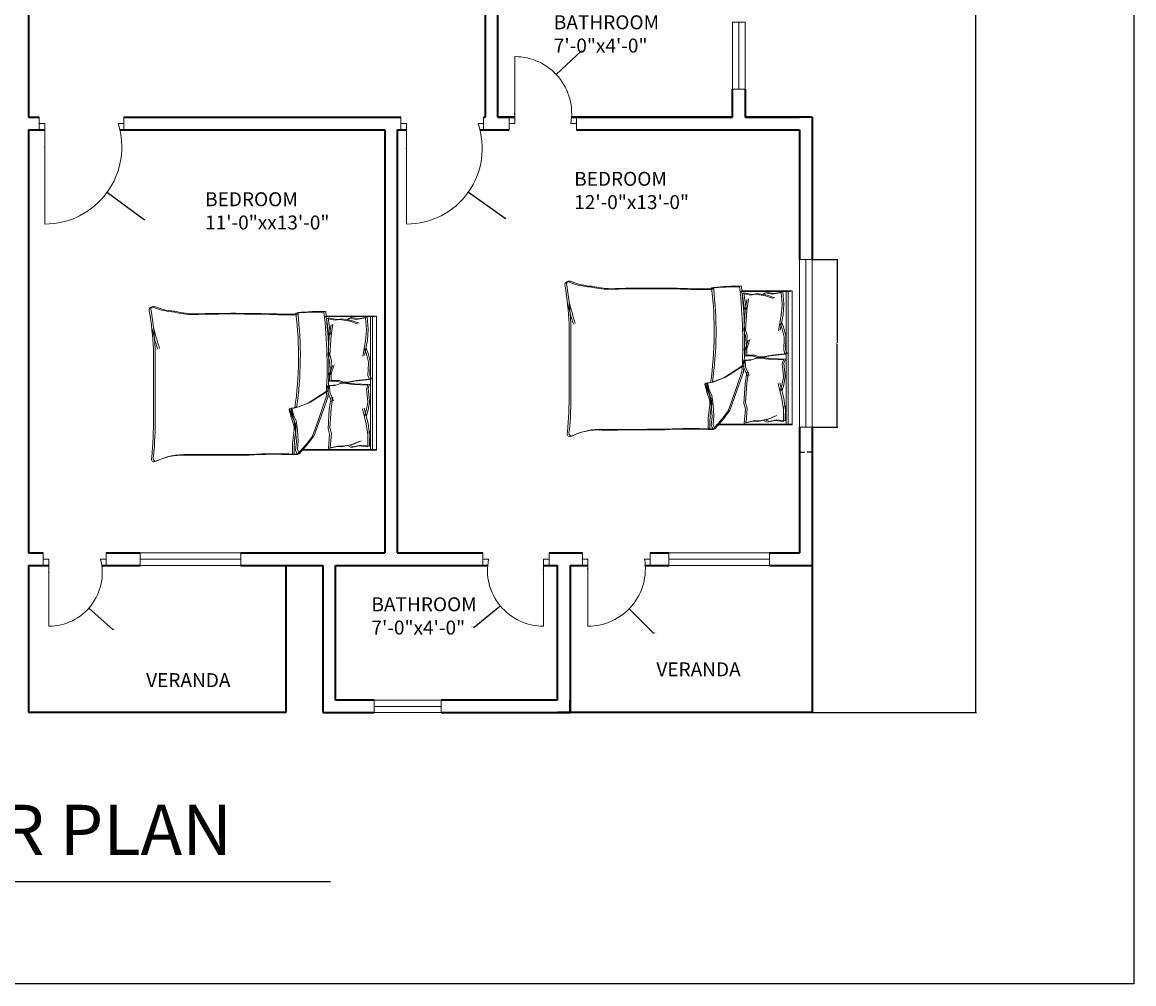
# Model space of a CAD drawing. Units: inches. Extents: x 2163 to 2982, y 1024 to 2288.
# Tile 5 of 22: x 2585 to 2982, y 1046 to 1390. Entities that reach past the tile are written whole.
import ezdxf

# ---------------------------------------------------------------- set-up
doc = ezdxf.new("R2010")
doc.units = ezdxf.units.IN
for name, color, linetype, lineweight in [('A-ANNO-DIMS', 2, 'Continuous', 18), ('A-ANNO-TTLB', 7, 'Continuous', 25), ('A-AREA-IDEN', 7, 'Continuous', 18), ('A-DOOR', 11, 'Continuous', 18), ('A-FURN', 8, 'Continuous', 13), ('A-GLAZ', 161, 'Continuous', 18), ('A-WALL', 7, 'Continuous', 35)]:
    doc.layers.add(name, color=color, linetype=linetype, lineweight=lineweight)
doc.styles.get("Standard").update_dxf_attribs({"font": 'arial.ttf'})
doc.dimstyles.get("Standard").update_dxf_attribs({"dimtxt": 0.18, "dimasz": 0.18, "dimexe": 0.18, "dimexo": 0.0625, "dimgap": 0.09, "dimtad": 0, "dimtih": 1, "dimtoh": 1, "dimdec": 4, "dimzin": 0, "dimdsep": 46, "dimtxsty": 'Standard', "dimcen": 0.09, "dimadec": 0, "dimazin": 0, "dimtfac": 1, "dimtdec": 4, "dimtofl": 0, "dimtmove": 0, "dimatfit": 3, "dimfxl": 1, "dimtolj": 1, "dimtzin": 0, "dimarcsym": 0})

# ---------------------------------------------------------------- blocks, each defined once
blk = doc.blocks.new('BED-DOUBLE')
for p, q in [((27.75, 52.87), (24.5, 49.16)), ((27.75, 52.87), (24.5, 49.16)), ((28.38, 53.1), (25.13, 49.39)), ((28.38, 53.1), (25.13, 49.39)), ((29.49, 52.95), (27.75, 52.87, 3.87)), ((29.49, 52.95), (27.75, 52.87, 3.87)), ((28.36, 51.33), (27.75, 52.87)), ((28.36, 51.33), (27.75, 52.87)), ((30.13, 53.18), (28.38, 53.1, 3.87)), ((29, 51.56), (28.38, 53.1)), ((30.13, 53.18), (28.38, 53.1, 3.87)), ((29, 51.56), (28.38, 53.1)), ((0, 51.49), (0.64, 51.49)), ((0, 3.47), (0, 51.49)), ((0, 51.27), (26.61, 51.27)), ((0, 51.27), (26.61, 51.27)), ((0.64, 51.49), (27.25, 51.49)), ((0.64, 51.49), (27.25, 51.49)), ((1.53, 3.48), (1.53, 51.27)), ((1.53, 3.47), (1.53, 51.27)), ((2.17, 3.7), (2.17, 51.49)), ((2.17, 3.7), (2.17, 51.49)), ((2.56, 50.11), (2.46, 44.71)), ((2.56, 50.11), (2.46, 44.71)), ((2.56, 50.11), (5.77, 49.73)), ((2.56, 50.11), (5.77, 49.73)), ((3.2, 50.34), (3.1, 44.94)), ((3.2, 50.34), (3.1, 44.94)), ((3.2, 50.34), (6.41, 49.96)), ((3.2, 50.34), (6.41, 49.96)), ((8.26, 49.31), (5.58, 48.13)), ((8.26, 49.31), (5.58, 48.13)), ((5.77, 49.73), (8.34, 50.33)), ((5.77, 49.73), (8.34, 50.33)), ((8.9, 49.54), (6.22, 48.36)), ((8.9, 49.54), (6.22, 48.36)), ((6.41, 49.96), (8.98, 50.56)), ((6.41, 49.96), (8.98, 50.56)), ((11.83, 50.11), (8.26, 49.31)), ((11.83, 50.11), (8.26, 49.31)), ((8.34, 50.33), (9.38, 49.81)), ((8.34, 50.33), (9.38, 49.81)), ((12.47, 50.34), (8.9, 49.54)), ((12.47, 50.34), (8.9, 49.54)), ((8.98, 50.56), (10.02, 50.04)), ((8.98, 50.56), (10.02, 50.04)), ((13.43, 49.92), (11.83, 50.11)), ((13.43, 49.92), (11.83, 50.11)), ((14.07, 50.15), (12.47, 50.34)), ((14.07, 50.15), (12.47, 50.34)), ((16.57, 50.7), (13.43, 49.92)), ((16.57, 50.7), (13.43, 49.92)), ((17.21, 50.93), (14.07, 50.15)), ((17.21, 50.93), (14.07, 50.15)), ((16.17, 45.57), (16.57, 50.7)), ((16.17, 45.57), (16.57, 50.7)), ((16.81, 45.79), (17.21, 50.93)), ((16.81, 45.79), (17.21, 50.93)), ((24.5, 49.16), (22.33, 46.22)), ((24.5, 49.16), (22.33, 46.22)), ((25.13, 49.39), (22.97, 46.45)), ((25.13, 49.39), (22.97, 46.45)), ((28.06, 48.23), (28.36, 51.33)), ((28.06, 48.23), (28.36, 51.33)), ((28.36, 44.36), (28.06, 48.23)), ((28.36, 44.36), (28.06, 48.23)), ((28.69, 48.46), (29, 51.56)), ((28.69, 48.46), (29, 51.56)), ((29, 44.59), (28.69, 48.46)), ((29, 44.59), (28.69, 48.46)), ((2.46, 44.71), (2.54, 45.71)), ((2.46, 44.71), (2.54, 45.71)), ((2.54, 45.71), (3.07, 41.91)), ((2.54, 45.71), (3.07, 41.91)), ((3.1, 44.94), (3.18, 45.94)), ((3.1, 44.94), (3.18, 45.94)), ((3.18, 45.94), (3.71, 42.14)), ((3.18, 45.94), (3.71, 42.14)), ((16.73, 43.61), (16.17, 45.57)), ((16.73, 43.61), (16.17, 45.57)), ((17.37, 43.83), (16.81, 45.79)), ((17.37, 43.83), (16.81, 45.79)), ((16.93, 36.82), (17.37, 43.83)), ((16.93, 36.82), (17.37, 43.83)), ((22.33, 46.22), (20.32, 40.64)), ((22.33, 46.22), (20.32, 40.64)), ((22.97, 46.45), (20.96, 40.87)), ((22.97, 46.45), (20.96, 40.87)), ((28.83, 40.95), (28.36, 44.36)), ((28.83, 40.95), (28.36, 44.36)), ((29.47, 41.18), (29, 44.59)), ((29.47, 41.18), (29, 44.59)), ((3.07, 41.91), (4.42, 36.49)), ((3.07, 41.91), (4.42, 36.49)), ((3.71, 42.14), (5.06, 36.72)), ((3.71, 42.14), (5.06, 36.72)), ((16.29, 36.6), (16.73, 43.61)), ((16.29, 36.6), (16.73, 43.61)), ((20.32, 40.64), (17.38, 32.31)), ((20.32, 40.64), (17.38, 32.31)), ((20.96, 40.87), (18.02, 32.53)), ((20.96, 40.87), (18.02, 32.53)), ((29.76, 38.94), (28.83, 40.95)), ((29.76, 38.94), (28.83, 40.95)), ((30.4, 39.17), (29.47, 41.18)), ((30.4, 39.17), (29.47, 41.18)), ((79.88, 15.29), (79.88, 39.91)), ((79.88, 15.29), (79.88, 39.91)), ((3.08, 37.14), (2.54, 34.2)), ((3.08, 37.13), (2.54, 34.2)), ((3.67, 39.2), (3.08, 37.14)), ((3.67, 39.2), (3.08, 37.13)), ((3.72, 37.36), (3.18, 34.43)), ((3.72, 37.36), (3.18, 34.43)), ((4.31, 39.43), (3.72, 37.36)), ((4.31, 39.43), (3.72, 37.36)), ((15.63, 32.56), (16.29, 36.6)), ((15.63, 32.56), (16.29, 36.6)), ((16.27, 32.79), (16.93, 36.82)), ((16.27, 32.79), (16.93, 36.82)), ((23.88, 34.45), (28.36, 36.15)), ((23.88, 34.45), (28.36, 36.15)), ((24.52, 34.68), (29, 36.38)), ((24.52, 34.68), (29, 36.38)), ((28.36, 36.15), (30.38, 36.46)), ((28.36, 36.15), (30.38, 36.46)), ((29, 36.38), (31.02, 36.69)), ((29, 36.38), (31.02, 36.69)), ((30.38, 36.46), (29.76, 38.94)), ((30.38, 36.46), (29.76, 38.94)), ((31.02, 36.69), (30.4, 39.17)), ((31.02, 36.69), (30.4, 39.17)), ((79.24, 15.06), (79.24, 39.68)), ((79.24, 15.06), (79.24, 39.68)), ((2.54, 34.2), (2.56, 33.88)), ((2.54, 34.2), (2.56, 33.88)), ((2.56, 33.88), (2.98, 29.46)), ((2.56, 33.88), (2.98, 29.46)), ((3.18, 34.43), (3.2, 34.11)), ((3.18, 34.43), (3.2, 34.11)), ((3.2, 34.11), (3.62, 29.68)), ((3.2, 34.11), (3.62, 29.68)), ((16.74, 30.75), (15.45, 33.82)), ((16.74, 30.75), (15.45, 33.82)), ((17.38, 30.98), (16.09, 34.05)), ((17.38, 30.98), (16.09, 34.05)), ((17.38, 30.26), (23.88, 34.45)), ((17.38, 30.26), (23.88, 34.45)), ((18.02, 30.49), (24.52, 34.68)), ((18.02, 30.49), (24.52, 34.68)), ((2.98, 29.46), (2.49, 27.98)), ((2.98, 29.46), (2.49, 27.98)), ((2.49, 27.98), (7.87, 27.73)), ((2.49, 27.98), (7.87, 27.73)), ((3.62, 29.68), (3.13, 28.21)), ((3.62, 29.68), (3.13, 28.2)), ((3.13, 28.21), (8.51, 27.96)), ((3.13, 28.2), (8.51, 27.96)), ((8.51, 27.96), (11.72, 27.58)), ((8.51, 27.96), (11.72, 27.58)), ((12.38, 27.44), (14.22, 28.13)), ((12.38, 27.44), (14.22, 28.13)), ((13.02, 27.66), (14.86, 28.36)), ((13.02, 27.66), (14.86, 28.36)), ((14.22, 28.13), (16.89, 28.3)), ((14.22, 28.13), (16.89, 28.3)), ((14.86, 28.36), (17.53, 28.53)), ((14.86, 28.36), (17.53, 28.53)), ((16.89, 28.3), (16.74, 30.75)), ((16.89, 28.3), (16.74, 30.75)), ((17.53, 28.53), (17.38, 30.98)), ((17.53, 28.53), (17.38, 30.98)), ((1.87, 25.98), (7.22, 26.56)), ((1.87, 25.98), (7.22, 26.56)), ((2.45, 24.54), (1.87, 25.98)), ((2.45, 24.54), (1.87, 25.98)), ((2.3, 20.09), (2.45, 24.54)), ((2.3, 20.09), (2.45, 24.54)), ((2.51, 26.21), (7.86, 26.79)), ((2.51, 26.21), (7.86, 26.79)), ((3.09, 24.77), (2.51, 26.21)), ((3.09, 24.77), (2.51, 26.21)), ((2.94, 20.32), (3.09, 24.77)), ((2.94, 20.32), (3.09, 24.77)), ((7.22, 26.56), (10.4, 27.14)), ((7.22, 26.56), (10.4, 27.14)), ((7.86, 26.79), (11.04, 27.37)), ((7.86, 26.79), (11.04, 27.37)), ((7.87, 27.73), (11.08, 27.35)), ((7.87, 27.73), (11.08, 27.35)), ((10.4, 27.14), (11.7, 27.14)), ((10.4, 27.14), (11.7, 27.14)), ((11.04, 27.37), (12.34, 27.37)), ((11.04, 27.37), (12.34, 27.37)), ((11.08, 27.35), (12.38, 27.44)), ((11.08, 27.35), (12.38, 27.44)), ((11.7, 27.14), (13.58, 26.56)), ((11.7, 27.14), (13.58, 26.56)), ((11.72, 27.58), (13.02, 27.66)), ((11.72, 27.58), (13.02, 27.66)), ((12.34, 27.37), (14.22, 26.79)), ((12.34, 27.37), (14.22, 26.79)), ((13.58, 26.56), (16.26, 26.56)), ((13.58, 26.56), (16.26, 26.56)), ((14.22, 26.79), (16.9, 26.79)), ((14.22, 26.79), (16.9, 26.79)), ((16.26, 24.1), (15.17, 20.96)), ((16.26, 24.1), (15.17, 20.96)), ((16.9, 24.33), (15.81, 21.19)), ((16.9, 24.33), (15.81, 21.19)), ((16.17, 19.38), (16.57, 24.52)), ((16.17, 19.38), (16.57, 24.52)), ((16.26, 26.56), (16.26, 24.1)), ((16.26, 26.56), (16.26, 24.1)), ((16.81, 19.61), (17.21, 24.74)), ((16.81, 19.61), (17.21, 24.74)), ((16.9, 26.79), (16.9, 24.33)), ((16.9, 26.79), (16.9, 24.33)), ((2.3, 19.77), (2.3, 20.09)), ((2.3, 19.77), (2.3, 20.09)), ((2.94, 20), (2.94, 20.32)), ((2.94, 20), (2.94, 20.32)), ((3.67, 17.11), (2.94, 20)), ((3.67, 17.11), (2.94, 20)), ((3.03, 16.88), (2.3, 19.77)), ((3.03, 16.88), (2.3, 19.77)), ((3.75, 14.85), (3.03, 16.88)), ((3.75, 14.85), (3.03, 16.88)), ((3.32, 12.11), (4.33, 17.6)), ((3.32, 12.11), (4.33, 17.6)), ((4.39, 15.08), (3.67, 17.11)), ((4.39, 15.08), (3.67, 17.11)), ((3.96, 12.34), (4.97, 17.83)), ((3.96, 12.34), (4.97, 17.83)), ((16.73, 17.42), (16.17, 19.38)), ((16.73, 17.42), (16.17, 19.38)), ((16.29, 10.41), (16.73, 17.42)), ((16.29, 10.41), (16.73, 17.42)), ((17.37, 17.65), (16.81, 19.61)), ((17.37, 17.65), (16.81, 19.61)), ((16.93, 10.64), (17.37, 17.65)), ((16.93, 10.64), (17.37, 17.65)), ((3.03, 8.28), (3.32, 12.11)), ((3.03, 8.28), (3.32, 12.11)), ((3.67, 8.51), (3.96, 12.34)), ((3.67, 8.51), (3.96, 12.34)), ((3.01, 8.18), (3.03, 8.28)), ((3.01, 8.18), (3.03, 8.28)), ((3.34, 3.9), (3.01, 8.18)), ((3.34, 3.9), (3.01, 8.18)), ((3.65, 8.41), (3.67, 8.51)), ((3.65, 8.41), (3.67, 8.51)), ((3.98, 4.13), (3.65, 8.41)), ((3.98, 4.13), (3.65, 8.41)), ((15.63, 6.38), (16.29, 10.41)), ((15.63, 6.38), (16.29, 10.41)), ((16.27, 6.61), (16.93, 10.64)), ((16.27, 6.61), (16.93, 10.64)), ((16.29, 10.41), (16.62, 9.28)), ((16.29, 10.41), (16.62, 9.28)), ((16.62, 9.28), (17.34, 4.18)), ((16.62, 9.28), (17.34, 4.18)), ((16.93, 10.64), (17.26, 9.51)), ((16.93, 10.64), (17.26, 9.51)), ((17.26, 9.51), (17.98, 4.41)), ((17.26, 9.51), (17.98, 4.41)), ((3.32, 3.89), (6.5, 4.47)), ((3.32, 3.89), (6.5, 4.47)), ((3.96, 4.12), (7.14, 4.7)), ((3.96, 4.12), (7.14, 4.7)), ((8.95, 5.05), (6.21, 6.06)), ((8.95, 5.05), (6.21, 6.06)), ((6.5, 4.47), (9.1, 4.04)), ((6.5, 4.47), (9.1, 4.04)), ((9.59, 5.28), (6.85, 6.29)), ((9.59, 5.28), (6.85, 6.29)), ((7.14, 4.7), (9.74, 4.27)), ((7.14, 4.7), (9.74, 4.27)), ((12.57, 4.47), (8.95, 5.05)), ((12.57, 4.47), (8.95, 5.05)), ((9.1, 4.04), (10.11, 4.62)), ((9.1, 4.04), (10.11, 4.62)), ((13.21, 4.7), (9.59, 5.28)), ((13.21, 4.7), (9.59, 5.28)), ((9.74, 4.27), (10.75, 4.85)), ((9.74, 4.27), (10.75, 4.85)), ((14.16, 4.76), (12.57, 4.47)), ((14.16, 4.76), (12.57, 4.47)), ((14.8, 4.99), (13.21, 4.7)), ((14.8, 4.99), (13.21, 4.7)), ((17.34, 4.18), (14.16, 4.76)), ((17.34, 4.18), (14.16, 4.76)), ((17.98, 4.41), (14.8, 4.99)), ((17.98, 4.41), (14.8, 4.99)), ((18.11, 3.48), (0, 3.48)), ((18.11, 3.47), (0, 3.47)), ((18.75, 3.7), (0.64, 3.7)), ((18.75, 3.7), (0.64, 3.7))]:
    blk.add_line(p, q)
for centre, radius, start, end in [((69.31, 76.39), 23.07, 267.4714, 296.4681), ((69.31, 76.39), 23.07, 267.4714, 296.4681), ((79.51, 54.64), 1.1, 332.6588, 86.02), ((79.51, 54.64), 1.1, 332.6588, 86.02), ((-6.66, 51.33), 36.18, 349.8763, 2.5657), ((-6.66, 51.33), 36.18, 349.8763, 2.5657), ((36.31, 182.27), 129.5, 266.9791, 273.8365), ((36.31, 182.27), 129.5, 266.9791, 273.8365), ((-6.02, 51.56), 36.18, 349.8763, 2.5657), ((-6.02, 51.56), 36.18, 349.8763, 2.5657), ((36.95, 182.49), 129.5, 266.9791, 273.8365), ((36.95, 182.49), 129.5, 266.9791, 273.8365), ((67.82, -4508.74), 4561.86, 90.00217, 90.28689), ((67.82, -4508.74), 4561.86, 90.00217, 90.28689), ((68.46, -4508.52), 4561.86, 90.00217, 90.28689), ((68.46, -4508.52), 4561.86, 90.00217, 90.28689), ((68.67, 76.16), 23.07, 267.4714, 296.4681), ((68.67, 76.16), 23.07, 267.4714, 296.4681), ((78.87, 54.41), 1.1, 332.6588, 86.02), ((78.87, 54.41), 1.1, 332.6588, 86.02), ((212.28, 41.15), 133.04, 174.4998, 180.6351), ((212.28, 41.15), 133.04, 174.4998, 180.6351), ((212.92, 41.38), 133.04, 174.4998, 180.6351), ((212.92, 41.38), 133.04, 174.4998, 180.6351), ((35.07, 43.74), 6.22, 168.6608, 203.7384), ((35.07, 43.74), 6.22, 168.6608, 203.7384), ((35.71, 43.97), 6.22, 168.6608, 203.7384), ((35.71, 43.97), 6.22, 168.6608, 203.7384), ((1.48, 31.15), 29.65, 10.6617, 19.8806), ((1.48, 31.15), 29.65, 10.6617, 19.8806), ((2.12, 31.38), 29.65, 10.6617, 19.8806), ((2.12, 31.38), 29.65, 10.6617, 19.8806), ((156.32, 17.76), 129.02, 171.7845, 186.9006), ((156.32, 17.76), 129.02, 171.7845, 186.9006), ((156.96, 17.98), 129.02, 171.7845, 186.9006), ((156.96, 17.98), 129.02, 171.7845, 186.9006), ((30.44, 36.64), 0.185, 250.2464, 1.1377), ((30.44, 36.64), 0.185, 250.2464, 1.1377), ((31.08, 36.86), 0.185, 250.2464, 1.1377), ((31.08, 36.86), 0.185, 250.2464, 1.1377), ((182.05, 21.36), 164.97, 176.0865, 186.7821), ((182.05, 21.36), 164.97, 176.0865, 186.7821), ((182.69, 21.59), 164.97, 176.0865, 186.7821), ((182.69, 21.59), 164.97, 176.0865, 186.7821), ((-23.71, -17.22), 106.46, 13.3832, 17.7053), ((-23.71, -17.22), 106.46, 13.3832, 17.7053), ((-23.07, -16.99), 106.46, 13.3832, 17.7053), ((-23.07, -16.99), 106.46, 13.3832, 17.7053), ((200.84, 21.43), 121.76, 182.9958, 189.4091), ((200.84, 21.43), 121.76, 182.9958, 189.4091), ((201.48, 21.66), 121.76, 182.9958, 189.4091), ((201.48, 21.65), 121.76, 182.9958, 189.4091), ((20.1, 85.16), 83.31, 268.7218, 275.604), ((20.1, 85.16), 83.31, 268.7218, 275.604), ((20.74, 85.39), 83.31, 268.7218, 275.604), ((20.74, 85.39), 83.31, 268.7218, 275.604), ((31.17, -167.31), 170.11, 88.4762, 91.0082), ((31.17, -167.31), 170.11, 88.4762, 91.0082), ((31.81, -167.08), 170.11, 88.4762, 91.0082), ((31.81, -167.08), 170.11, 88.4762, 91.0082), ((50.61, 484.82), 482.31, 268.2277, 271.7185), ((50.61, 484.82), 482.31, 268.2277, 271.7185), ((51.25, 485.05), 482.31, 268.2277, 271.7185), ((51.25, 485.05), 482.31, 268.2277, 271.7185), ((64.51, -26.9), 29.63, 76.0648, 88.9113), ((64.51, -26.9), 29.63, 76.0648, 88.9113), ((65.15, -26.67), 29.63, 76.0648, 88.9113), ((65.15, -26.67), 29.63, 76.0648, 88.9113), ((70.28, -21.66), 23.56, 67.9751, 86.652), ((70.28, -21.66), 23.56, 67.9751, 86.652), ((70.91, -21.43), 23.56, 67.9751, 86.652), ((70.91, -21.43), 23.56, 67.9751, 86.652), ((79.72, 1.09), 1.09, 236.1736, 23.4781), ((79.72, 1.09), 1.09, 236.1736, 23.4781), ((80.36, 1.32), 1.09, 236.1736, 23.4781), ((80.36, 1.32), 1.09, 236.1736, 23.4781)]:
    blk.add_arc(centre, radius, start, end)
blk = doc.blocks.new('WIN-24')
for p, q in [((0, 24), (4.5, 24)), ((0, 24), (0, 0)), ((4.5, 24), (2.25, 24)), ((2.25, 24), (2.25, 0)), ((4.5, 24), (4.5, 0)), ((2.25, 0), (0, 0)), ((0, 0), (4.5, 0))]:
    blk.add_line(p, q)
blk = doc.blocks.new('WIN-60')
for p, q in [((2.25, 60), (0, 60)), ((0, 60), (4.5, 60)), ((0, 60), (0, 0)), ((2.25, 0), (2.25, 60)), ((4.5, 60), (4.5, 0)), ((0, 0), (4.5, 0)), ((4.5, 0), (2.25, 0))]:
    blk.add_line(p, q)
blk = doc.blocks.new('WIN-36')
for p, q in [((2.25, 36), (0, 36)), ((0, 36), (4.5, 36)), ((0, 36), (0, 0)), ((2.25, 0), (2.25, 36)), ((4.5, 36), (4.5, 0)), ((0, 0), (4.5, 0)), ((4.5, 0), (2.25, 0))]:
    blk.add_line(p, q)
blk = doc.blocks.new('*D13')
at = {"layer": 'A-ANNO-DIMS', "color": 0, "lineweight": -2, "transparency": 16777216}
for p, q in [((2867.4, 1305.36), (2876.52, 1305.36)), ((2876.34, 1305.18), (2876.34, 1275.54)), ((2876.34, 1245.54), (2876.34, 1275.18)), ((2867.4, 1245.36), (2876.52, 1245.36))]:
    blk.add_line(p, q, dxfattribs=at)
at = {"layer": 'A-ANNO-DIMS', "color": 0, "transparency": 16777216}
for points in [[(2876.31, 1305.18), (2876.37, 1305.18), (2876.34, 1305.36)], [(2876.31, 1245.54), (2876.37, 1245.54), (2876.34, 1245.36)]]:
    blk.add_solid(points, dxfattribs=at)
at = {"layer": 'Defpoints', "color": 0, "transparency": 16777216}
for p in [(2867.34, 1305.36), (2876.34, 1305.36), (2867.34, 1245.36)]:
    blk.add_point(p, dxfattribs=at)
at = {"layer": 'A-ANNO-DIMS', "color": 0, "transparency": 16777216, "insert": (2876.34, 1275.36), "char_height": 0.18, "attachment_point": 5}
blk.add_mtext('\\A1;WINDOW 60 TYP.', dxfattribs=at)
blk = doc.blocks.new('*D14')
at = {"layer": 'A-ANNO-DIMS', "color": 0, "lineweight": -2, "transparency": 16777216}
for p, q in [((2862.84, 1245.3), (2862.84, 1236.18)), ((2867.34, 1245.3), (2867.34, 1236.18)), ((2863.02, 1236.36), (2864.63, 1236.36)), ((2867.16, 1236.36), (2865.55, 1236.36))]:
    blk.add_line(p, q, dxfattribs=at)
at = {"layer": 'A-ANNO-DIMS', "color": 0, "transparency": 16777216}
for points in [[(2863.02, 1236.39), (2863.02, 1236.33), (2862.84, 1236.36)], [(2867.16, 1236.39), (2867.16, 1236.33), (2867.34, 1236.36)]]:
    blk.add_solid(points, dxfattribs=at)
at = {"layer": 'Defpoints', "color": 0, "transparency": 16777216}
for p in [(2862.84, 1245.36), (2867.34, 1245.36), (2867.34, 1236.36)]:
    blk.add_point(p, dxfattribs=at)
at = {"layer": 'A-ANNO-DIMS', "color": 0, "transparency": 16777216, "insert": (2865.09, 1236.36), "char_height": 0.18, "attachment_point": 5}
blk.add_mtext('\\A1;5 TYP.', dxfattribs=at)
blk = doc.blocks.new('*D32')
at = {"layer": 'A-ANNO-DIMS', "color": 0, "lineweight": -2, "transparency": 16777216}
for p, q in [((2867.4, 2229.27), (2926.17, 2229.27)), ((2925.99, 2229.09), (2925.99, 1686.35)), ((2925.99, 1143.25), (2925.99, 1685.99)), ((2867.4, 1143.07), (2926.17, 1143.07))]:
    blk.add_line(p, q, dxfattribs=at)
at = {"layer": 'A-ANNO-DIMS', "color": 0, "transparency": 16777216}
for points in [[(2925.96, 2229.09), (2926.02, 2229.09), (2925.99, 2229.27)], [(2925.96, 1143.25), (2926.02, 1143.25), (2925.99, 1143.07)]]:
    blk.add_solid(points, dxfattribs=at)
at = {"layer": 'Defpoints', "color": 0, "transparency": 16777216}
for p in [(2867.34, 2229.27), (2925.99, 2229.27), (2867.34, 1143.07)]:
    blk.add_point(p, dxfattribs=at)
at = {"layer": 'A-ANNO-DIMS', "color": 0, "transparency": 16777216, "insert": (2925.99, 1686.17), "char_height": 0.18, "attachment_point": 5}
blk.add_mtext('\\A1;1086.2', dxfattribs=at)
blk = doc.blocks.new('*D45')
at = {"layer": 'A-ANNO-DIMS', "color": 0, "lineweight": -2, "transparency": 16777216}
for p, q in [((2592.54, 1345.61), (2592.72, 1345.61)), ((2592.63, 1345.52), (2592.63, 1345.7)), ((2628.28, 1319.58), (2615.06, 1329.24)), ((2628.46, 1319.58), (2628.28, 1319.58))]:
    blk.add_line(p, q, dxfattribs=at)
at = {"layer": 'A-ANNO-DIMS', "color": 0, "transparency": 16777216}
blk.add_solid([(2615.08, 1329.26), (2615.04, 1329.21), (2614.91, 1329.34)], dxfattribs=at)
at = {"layer": 'Defpoints', "color": 0, "transparency": 16777216}
for p in [(2592.63, 1345.61), (2614.91, 1329.34)]:
    blk.add_point(p, dxfattribs=at)
at = {"layer": 'A-ANNO-DIMS', "color": 0, "transparency": 16777216, "insert": (2628.94, 1319.58), "char_height": 0.18, "attachment_point": 5}
blk.add_mtext('\\A1;R27.59', dxfattribs=at)
blk = doc.blocks.new('*D48')
at = {"layer": 'A-ANNO-DIMS', "color": 0, "lineweight": -2, "transparency": 16777216}
for p, q in [((2722.07, 1345.1), (2722.25, 1345.1)), ((2722.16, 1345.01), (2722.16, 1345.19)), ((2757.49, 1320), (2744.39, 1329.31)), ((2757.67, 1320), (2757.49, 1320))]:
    blk.add_line(p, q, dxfattribs=at)
at = {"layer": 'A-ANNO-DIMS', "color": 0, "transparency": 16777216}
blk.add_solid([(2744.4, 1329.34), (2744.37, 1329.29), (2744.24, 1329.42)], dxfattribs=at)
at = {"layer": 'Defpoints', "color": 0, "transparency": 16777216}
for p in [(2722.16, 1345.1), (2744.24, 1329.42)]:
    blk.add_point(p, dxfattribs=at)
at = {"layer": 'A-ANNO-DIMS', "color": 0, "transparency": 16777216, "insert": (2758.22, 1320), "char_height": 0.18, "attachment_point": 5}
blk.add_mtext('\\A1;R27.086', dxfattribs=at)
blk = doc.blocks.new('*D66')
at = {"layer": 'A-ANNO-DIMS', "color": 0, "lineweight": -2, "transparency": 16777216}
for p, q in [((2594, 1193.17), (2594.18, 1193.17)), ((2594.09, 1193.08), (2594.09, 1193.26)), ((2617.05, 1172.89), (2608.58, 1180.37)), ((2617.23, 1172.89), (2617.05, 1172.89))]:
    blk.add_line(p, q, dxfattribs=at)
at = {"layer": 'A-ANNO-DIMS', "color": 0, "transparency": 16777216}
blk.add_solid([(2608.6, 1180.4), (2608.56, 1180.35), (2608.44, 1180.49)], dxfattribs=at)
at = {"layer": 'Defpoints', "color": 0, "transparency": 16777216}
for p in [(2594.09, 1193.17), (2608.44, 1180.49)]:
    blk.add_point(p, dxfattribs=at)
at = {"layer": 'A-ANNO-DIMS', "color": 0, "transparency": 16777216, "insert": (2617.72, 1172.89), "char_height": 0.18, "attachment_point": 5}
blk.add_mtext('\\A1;R19.15', dxfattribs=at)
blk = doc.blocks.new('*D67')
at = {"layer": 'A-ANNO-DIMS', "color": 0, "lineweight": -2, "transparency": 16777216}
for p, q in [((2771.13, 1194.12), (2771.31, 1194.12)), ((2771.22, 1194.03), (2771.22, 1194.21)), ((2746.35, 1173.73), (2755.54, 1181.26)), ((2746.17, 1173.73), (2746.35, 1173.73))]:
    blk.add_line(p, q, dxfattribs=at)
at = {"layer": 'A-ANNO-DIMS', "color": 0, "transparency": 16777216}
blk.add_solid([(2755.52, 1181.29), (2755.56, 1181.24), (2755.68, 1181.38)], dxfattribs=at)
at = {"layer": 'Defpoints', "color": 0, "transparency": 16777216}
for p in [(2771.22, 1194.12), (2755.68, 1181.38)]:
    blk.add_point(p, dxfattribs=at)
at = {"layer": 'A-ANNO-DIMS', "color": 0, "transparency": 16777216, "insert": (2745.62, 1173.73), "char_height": 0.18, "attachment_point": 5}
blk.add_mtext('\\A1;R20.097', dxfattribs=at)
blk = doc.blocks.new('*D68')
at = {"layer": 'A-ANNO-DIMS', "color": 0, "lineweight": -2, "transparency": 16777216}
for p, q in [((2787, 1194.57), (2787.18, 1194.57)), ((2787.09, 1194.48), (2787.09, 1194.66)), ((2810.61, 1171.58), (2801.92, 1180.08)), ((2810.79, 1171.58), (2810.61, 1171.58))]:
    blk.add_line(p, q, dxfattribs=at)
at = {"layer": 'A-ANNO-DIMS', "color": 0, "transparency": 16777216}
blk.add_solid([(2801.94, 1180.1), (2801.9, 1180.06), (2801.79, 1180.2)], dxfattribs=at)
at = {"layer": 'Defpoints', "color": 0, "transparency": 16777216}
for p in [(2787.09, 1194.57), (2801.79, 1180.2)]:
    blk.add_point(p, dxfattribs=at)
at = {"layer": 'A-ANNO-DIMS', "color": 0, "transparency": 16777216, "insert": (2811.34, 1171.58), "char_height": 0.18, "attachment_point": 5}
blk.add_mtext('\\A1;R20.556', dxfattribs=at)
blk = doc.blocks.new('*D77')
at = {"layer": 'A-ANNO-DIMS', "color": 0, "lineweight": -2, "transparency": 16777216}
for p, q in [((2784.62, 1380.01), (2775.84, 1371.74)), ((2784.8, 1380.01), (2784.62, 1380.01)), ((2760.78, 1357.62), (2760.96, 1357.62)), ((2760.87, 1357.53), (2760.87, 1357.71))]:
    blk.add_line(p, q, dxfattribs=at)
at = {"layer": 'A-ANNO-DIMS', "color": 0, "transparency": 16777216}
blk.add_solid([(2775.82, 1371.76), (2775.86, 1371.72), (2775.71, 1371.62)], dxfattribs=at)
at = {"layer": 'Defpoints', "color": 0, "transparency": 16777216}
for p in [(2775.71, 1371.62), (2760.87, 1357.62)]:
    blk.add_point(p, dxfattribs=at)
at = {"layer": 'A-ANNO-DIMS', "color": 0, "transparency": 16777216, "insert": (2785.21, 1380.01), "char_height": 0.18, "attachment_point": 5}
blk.add_mtext('\\A1;R20.4', dxfattribs=at)

msp = doc.modelspace()

# ---------------------------------------------------------------- linework, layer by layer
at = {"layer": 'A-ANNO-TTLB'}
msp.add_line((2427.5046, 1082.6234), (2694.9452, 1082.6234), dxfattribs=at)
msp.add_lwpolyline([(2162.6841, 2274.6054), (2982.469, 2274.6054), (2982.469, 1045.9691), (2162.6841, 1045.9691)], close=True, dxfattribs=at)
at = {"layer": 'A-DOOR'}
for p, q in [((2760.8716, 1354.0188), (2760.8716, 1378.0188)), ((2590.6292, 1351.7688), (2590.6292, 1356.2688)), ((2590.6292, 1356.2688), (2590.6292, 1354.0188)), ((2590.6292, 1354.0188), (2592.6292, 1354.0188)), ((2592.6292, 1354.0188), (2592.6292, 1318.0188)), ((2620.9043, 1354.0188), (2618.9043, 1354.0188)), ((2620.9043, 1356.2688), (2620.9043, 1351.7688)), ((2620.9043, 1351.7688), (2620.9043, 1354.0188)), ((2720.1594, 1351.7688), (2720.1594, 1356.2688)), ((2720.1594, 1356.2688), (2720.1594, 1354.0188)), ((2720.1594, 1354.0188), (2722.1594, 1354.0188)), ((2722.1594, 1354.0188), (2722.1594, 1318.0188)), ((2749.7366, 1354.0188), (2747.7366, 1354.0188)), ((2749.7366, 1356.2688), (2749.7366, 1351.7688)), ((2749.7366, 1351.7688), (2749.7366, 1354.0188)), ((2758.8716, 1356.2688), (2758.8716, 1351.7688)), ((2758.8716, 1351.7688), (2758.8716, 1354.0188)), ((2758.8716, 1354.0188), (2760.8716, 1354.0188)), ((2782.9533, 1354.0188), (2780.9533, 1354.0188)), ((2782.9533, 1356.2688), (2782.9533, 1351.7688)), ((2782.9533, 1351.7688), (2782.9533, 1354.0188)), ((2592.0869, 1200.2688), (2592.0869, 1195.7688)), ((2592.0869, 1195.7688), (2592.0869, 1198.0188)), ((2592.0869, 1198.0188), (2594.0869, 1198.0188)), ((2594.0869, 1198.0188), (2594.0869, 1174.0188)), ((2614.6146, 1198.0188), (2612.6146, 1198.0188)), ((2614.6146, 1200.2688), (2614.6146, 1195.7688)), ((2614.6146, 1195.7688), (2614.6146, 1198.0188)), ((2749.508, 1195.7688), (2749.508, 1200.2688)), ((2749.508, 1200.2688), (2749.508, 1198.0188)), ((2749.508, 1198.0188), (2751.508, 1198.0188)), ((2773.2218, 1198.0188), (2771.2218, 1198.0188)), ((2771.2218, 1198.0188), (2771.2218, 1174.0188)), ((2773.2218, 1195.7688), (2773.2218, 1200.2688)), ((2773.2218, 1200.2688), (2773.2218, 1198.0188)), ((2785.093, 1195.7688), (2785.093, 1200.2688)), ((2785.093, 1200.2688), (2785.093, 1198.0188)), ((2785.093, 1198.0188), (2787.093, 1198.0188)), ((2787.093, 1198.0188), (2787.093, 1174.0188)), ((2809.358, 1198.0188), (2807.358, 1198.0188)), ((2809.358, 1195.7688), (2809.358, 1200.2688)), ((2809.358, 1200.2688), (2809.358, 1198.0188))]:
    msp.add_line(p, q, dxfattribs=at)
for centre, radius, start, end in [((2760.8716, 1357.6173), 20.4016, 349.841009, 90), ((2592.6292, 1345.6075), 27.5886, 270, 17.751249), ((2722.1594, 1345.1049), 27.086, 270, 19.214067), ((2594.0869, 1193.1705), 19.1517, 270, 14.664329), ((2771.2218, 1194.1154), 20.0965, 168.799919, 270), ((2787.093, 1194.5745), 20.5557, 270, 9.646048)]:
    msp.add_arc(centre, radius, start, end, dxfattribs=at)
at = {"layer": 'A-WALL'}
for p, q in [((2586.8389, 1648.0603), (2586.8389, 1356.2688)), ((2750.3389, 1404.2688), (2750.3389, 1356.2688)), ((2754.8389, 1356.2688), (2754.8389, 1404.2688)), ((2838.8389, 1356.2688), (2838.8389, 1366.3249)), ((2843.3389, 1366.3249), (2843.3389, 1356.2688)), ((2586.8389, 1356.2688), (2590.6292, 1356.2688)), ((2620.9043, 1356.2688), (2714.3389, 1356.2688)), ((2714.3389, 1356.2688), (2720.1594, 1356.2688)), ((2749.7366, 1356.2688), (2750.3389, 1356.2688)), ((2754.8389, 1356.2688), (2760.8716, 1356.2688)), ((2760.8716, 1356.2688), (2754.8389, 1356.2688)), ((2838.8389, 1356.2688), (2781.2285, 1356.2688)), ((2781.2285, 1356.2688), (2838.8389, 1356.2688)), ((2867.3389, 1356.2688), (2843.3389, 1356.2688)), ((2843.3389, 1356.2688), (2862.8389, 1356.2688)), ((2867.3389, 1356.2688), (2867.3389, 1305.3618)), ((2586.8389, 1351.7688), (2586.8389, 1200.2688)), ((2586.8389, 1351.7688), (2592.6292, 1351.7688)), ((2619.521, 1351.7688), (2714.3389, 1351.7688)), ((2714.3389, 1351.7688), (2714.3389, 1200.2688)), ((2718.8389, 1351.7688), (2722.1594, 1351.7688)), ((2718.8389, 1351.7688), (2718.8389, 1200.2688)), ((2748.4128, 1351.7688), (2758.8716, 1351.7688)), ((2782.9533, 1351.7688), (2862.8389, 1351.7688)), ((2862.8389, 1351.7688), (2862.8389, 1305.3618)), ((2862.8389, 1245.3618), (2862.8389, 1200.2688)), ((2867.3389, 1245.3618), (2867.3389, 1195.7688)), ((2586.8389, 1200.2688), (2592.0869, 1200.2688)), ((2614.6146, 1200.2688), (2626.8098, 1200.2688)), ((2662.8098, 1200.2688), (2714.3389, 1200.2688)), ((2718.8389, 1200.2688), (2749.508, 1200.2688)), ((2773.2218, 1200.2688), (2785.093, 1200.2688)), ((2776.2464, 1200.2688), (2780.7464, 1200.2688)), ((2809.358, 1200.2688), (2816.0529, 1200.2688)), ((2852.0529, 1200.2688), (2862.8389, 1200.2688)), ((2586.8389, 1195.7688), (2586.8389, 1143.2688)), ((2586.8389, 1195.7688), (2594.0869, 1195.7688)), ((2613.0614, 1195.7688), (2626.8098, 1195.7688)), ((2662.8098, 1195.7688), (2692.2464, 1195.7688)), ((2679.0829, 1143.2688), (2679.0829, 1195.7688)), ((2692.2464, 1195.7688), (2692.2464, 1143.0732)), ((2696.7464, 1147.5732), (2696.7464, 1195.7688)), ((2696.7464, 1195.7688), (2751.1934, 1195.7688)), ((2771.2218, 1195.7688), (2776.2464, 1195.7688)), ((2776.2464, 1147.5732), (2776.2464, 1195.7688)), ((2780.7464, 1195.7688), (2780.7464, 1143.0732)), ((2780.7464, 1195.7688), (2787.093, 1195.7688)), ((2807.6139, 1195.7688), (2816.0529, 1195.7688)), ((2852.0529, 1195.7688), (2867.3389, 1195.7688)), ((2867.3389, 1195.7688), (2867.3389, 1143.0732)), ((2710.5865, 1147.5732), (2696.7464, 1147.5732)), ((2776.2464, 1147.5732), (2734.5865, 1147.5732)), ((2780.7464, 1143.0732), (2780.7464, 1147.5732)), ((2586.8389, 1143.2688), (2679.0829, 1143.2688)), ((2692.2464, 1143.0732), (2710.5865, 1143.0732)), ((2734.5865, 1143.0732), (2776.2464, 1143.0732)), ((2780.7464, 1143.0732), (2776.2464, 1143.0732)), ((2776.2464, 1143.0732), (2780.7464, 1143.0732)), ((2867.3389, 1143.0732), (2780.7464, 1143.0732))]:
    msp.add_line(p, q, dxfattribs=at)

# ---------------------------------------------------------------- block references
at = {"layer": 'A-FURN', "rotation": 180}
for p in [(2860.2409, 1297.626), (2711.4412, 1288.5851)]:
    msp.add_blockref('BED-DOUBLE', p, dxfattribs=at)
at = {"layer": 'A-GLAZ', "extrusion": (0, 0, -1), "zscale": -1}
for p, rotation in [((-2838.839, 1390.3245), 180), ((-2710.587, 1143.0733), 90)]:
    msp.add_blockref('WIN-24', p, dxfattribs=dict(at, rotation=rotation))
at = {"layer": 'A-GLAZ'}
msp.add_blockref('WIN-60', (2862.839, 1245.3618), dxfattribs=at)
at = {"layer": 'A-GLAZ', "rotation": 270}
for p in [(2626.8094, 1200.2688), (2816.0525, 1200.2688)]:
    msp.add_blockref('WIN-36', p, dxfattribs=at)

# ---------------------------------------------------------------- texts
at = {"layer": 'A-ANNO-TTLB', "insert": (2442.4425, 1110.0829), "char_height": 18, "attachment_point": 1}
msp.add_mtext_dynamic_manual_height_columns('FIRST FLOOR PLAN', width=728.99492, gutter_width=12.5, heights=[0], dxfattribs=at)
at = {"layer": 'A-AREA-IDEN', "char_height": 5, "attachment_point": 1}
for s, width, insert in [('BATHROOM\\P7\'-0"x4\'-0"', 52.770015, (2774.8723, 1392.7938)), ('BEDROOM\\P12\'-0"x13\'-0"', 62.207874, (2782.1606, 1336.7403)), ('BEDROOM\\P11\'-0"xx13\'-0"', 110.183291, (2650.0452, 1329.4297)), ('BATHROOM\\P7\'-0"x4\'-0"', 77.436959, (2709.5926, 1184.369)), ('VERANDA', 68.460367, (2811.5789, 1161.0749)), ('VERANDA', 53.947048, (2628.9428, 1157.2097))]:
    msp.add_mtext_dynamic_manual_height_columns(s, width=width, gutter_width=12.5, heights=[0], dxfattribs=dict(at, insert=insert))

# ---------------------------------------------------------------- dimensions: what is measured, and where the dimension line sits
at = {"layer": 'A-ANNO-DIMS'}
dim = msp.add_linear_dim(base=(2925.9889, 2229.2688), p1=(2867.3389, 1143.0732), p2=(2867.3389, 2229.2688), angle=90, dimstyle='Standard', override={"dimdec": 1, "dimlfac": 1, "dimrnd": 0, "dimzin": 0, "dimdsep": 46, "dimlunit": 2}, dxfattribs=at)
dim.commit()
dim.dimension.update_dxf_attribs({"geometry": '*D32', "text_midpoint": (2925.9889, 1686.171)})
for center, mpoint, override, picture, middle in [((2760.8716, 1357.6173), (2775.713, 1371.6157), {"dimdec": 1, "dimlfac": 1, "dimrnd": 0, "dimzin": 0, "dimdsep": 46, "dimlunit": 2}, '*D77', (2785.2074, 1380.0148)), ((2592.6292, 1345.6075), (2614.9138, 1329.3431), {"dimdec": 2, "dimlfac": 1, "dimrnd": 0, "dimzin": 0, "dimdsep": 46, "dimlunit": 2}, '*D45', (2628.9446, 1319.5845)), ((2722.1594, 1345.1049), (2744.2398, 1329.4171), {"dimdec": 3, "dimlfac": 1, "dimrnd": 0, "dimzin": 0, "dimdsep": 46, "dimlunit": 2}, '*D48', (2758.2178, 1320.0045)), ((2771.2218, 1194.1154), (2755.6789, 1181.3761), {"dimdec": 3, "dimlfac": 1, "dimrnd": 0, "dimzin": 0, "dimdsep": 46, "dimlunit": 2}, '*D67', (2745.6234, 1173.7325)), ((2787.093, 1194.5745), (2801.791, 1180.2043), {"dimdec": 3, "dimlfac": 1, "dimrnd": 0, "dimzin": 0, "dimdsep": 46, "dimlunit": 2}, '*D68', (2811.3396, 1171.5822)), ((2594.0869, 1193.1705), (2608.4418, 1180.4929), {"dimdec": 2, "dimlfac": 1, "dimrnd": 0, "dimzin": 0, "dimdsep": 46, "dimlunit": 2}, '*D66', (2617.7153, 1172.8864))]:
    dim = msp.add_radius_dim(center=center, mpoint=mpoint, dimstyle='Standard', override=override, dxfattribs=at)
    dim.commit()
    dim.dimension.update_dxf_attribs({"geometry": picture, "text_midpoint": middle, "dimtype": 164})
dim = msp.add_linear_dim(base=(2876.3389, 1305.3618), p1=(2867.3389, 1245.3618), p2=(2867.3389, 1305.3618), angle=90, text='WINDOW <> TYP.', dimstyle='Standard', override={"dimdec": 0, "dimlfac": 1, "dimrnd": 0, "dimzin": 0, "dimdsep": 46, "dimlunit": 2}, dxfattribs=at)
dim.commit()
dim.dimension.update_dxf_attribs({"geometry": '*D13', "text_midpoint": (2876.3389, 1275.3618)})
dim = msp.add_linear_dim(base=(2867.3389150341, 1236.3618168908), p1=(2862.8389150341, 1245.3618168908), p2=(2867.3389150341, 1245.3618168908), text='<> TYP.', dimstyle='Standard', override={"dimdec": 0, "dimlfac": 1, "dimrnd": 0, "dimzin": 0, "dimdsep": 46, "dimlunit": 2}, dxfattribs=at)
dim.commit()
dim.dimension.update_dxf_attribs({"geometry": '*D14', "text_midpoint": (2865.0889150341, 1236.3618168908)})

doc.saveas('drawing.dxf')
